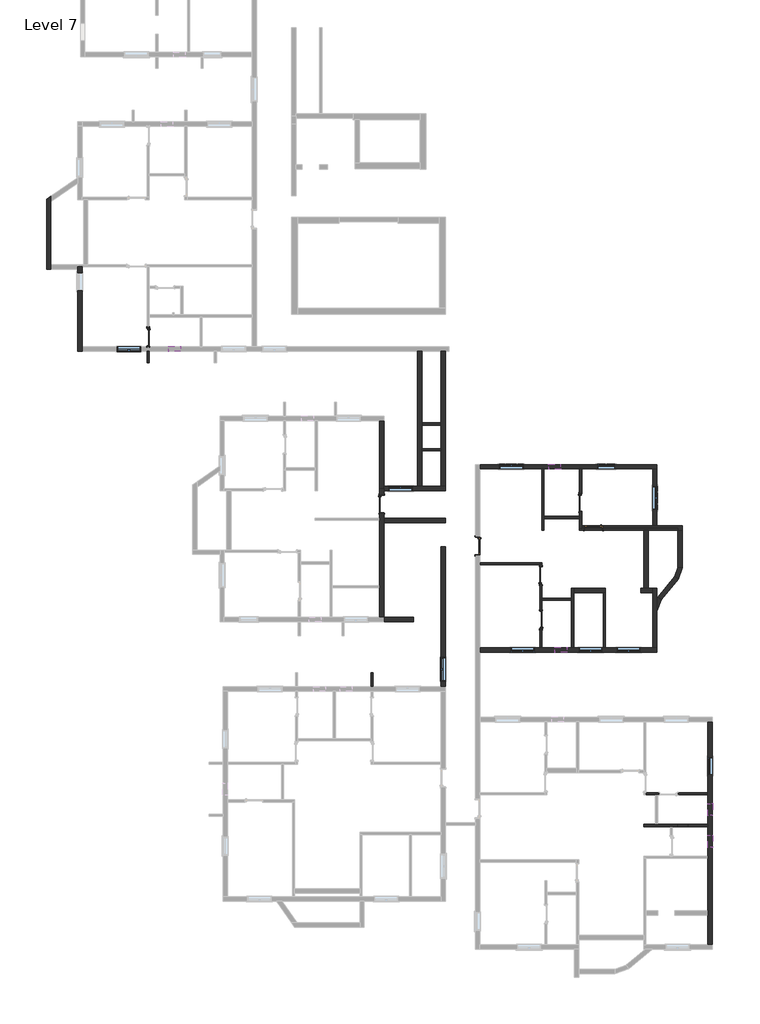
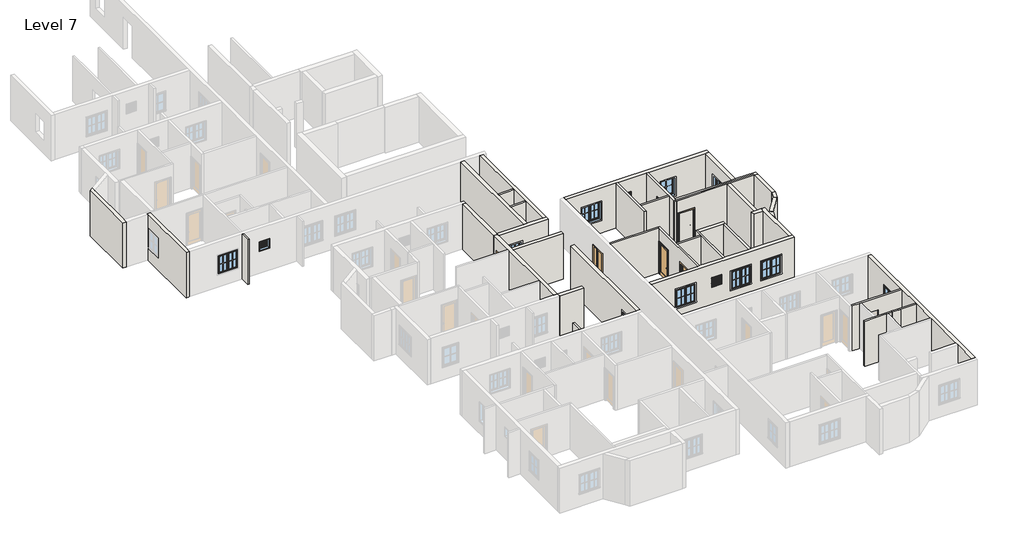
# One storey, part 3 of 7: 39 walls, 15 windows, 7 doors.
# Revit data of these elements (continued)
# Element 52 (IfcWindow, "Window-Casement-Double : 4' x 4'") (continued)
#   Interior Wall Closure = 0' - 2 1/4"
#   Frame Extension = 0' - 0 1/4"
#   Exterior Wall Closure = 0' - 1 1/4"
#   Interior Trim Visibility = yes
#   Exterior Trim Visibility = yes
#   Phase Created = New Construction
#   Materials on its faces: "Wood - Stained", "Glass", "Clad - White"
# Element 53 (IfcWindow, "Window-Casement-Double : 4' x 4'")
#   Mark = "176"
#   Window Inset = 0' - 0"
#   Interior Wall Closure = 0' - 2 1/4"
#   Frame Extension = 0' - 0 1/4"
#   Exterior Wall Closure = 0' - 1 1/4"
#   Interior Trim Visibility = yes
#   Exterior Trim Visibility = yes
#   Phase Created = New Construction
#   Materials on its faces: "Wood - Stained", "Glass", "Clad - White"
# Element 54 (IfcWindow, "Window-Casement-Double : 4' x 4'")
#   Mark = "187"
#   Window Inset = 0' - 0"
#   Interior Wall Closure = 0' - 2 1/4"
#   Frame Extension = 0' - 0 1/4"
#   Exterior Wall Closure = 0' - 1 1/4"
#   Interior Trim Visibility = yes
#   Exterior Trim Visibility = yes
#   Phase Created = New Construction
#   Materials on its faces: "Wood - Stained", "Glass", "Clad - White"
# Element 55 (IfcWindow, "Window-Casement-Double : 4' x 4'")
#   Mark = "190"
#   Window Inset = 0' - 0"
#   Interior Wall Closure = 0' - 2 1/4"
#   Frame Extension = 0' - 0 1/4"
#   Exterior Wall Closure = 0' - 1 1/4"
#   Interior Trim Visibility = yes
#   Exterior Trim Visibility = yes
#   Phase Created = New Construction
#   Materials on its faces: "Wood - Stained", "Glass", "Clad - White"
# Element 56 (IfcWindow, "Window-Casement-Double : 4' x 4'")
#   Mark = "195"
#   Window Inset = 0' - 0"
#   Interior Wall Closure = 0' - 2 1/4"
#   Frame Extension = 0' - 0 1/4"
#   Exterior Wall Closure = 0' - 1 1/4"
#   Interior Trim Visibility = yes
#   Exterior Trim Visibility = yes
#   Phase Created = New Construction
#   Materials on its faces: "Wood - Stained", "Glass", "Clad - White"
# Element 57 (IfcWindow, "Window-Louvers : 24\" x 24\"")
#   Mark = "138"
#   Blade Width = 1' - 10 1/2"
#   Phase Created = New Construction
#   Materials on its faces: "Birch"
# Element 58 (IfcWindow, "Window-Louvers : 24\" x 24\"")
#   Mark = "141"
#   Blade Width = 1' - 10 1/2"
#   Phase Created = New Construction
#   Materials on its faces: "Birch"
# Element 59 (IfcWindow, "Window-Louvers : 24\" x 24\"")
#   Mark = "142"
#   Blade Width = 1' - 10 1/2"
#   Phase Created = New Construction
#   Materials on its faces: "Birch"
# Element 60 (IfcWindow, "Window-Louvers : 24\" x 24\"")
#   Mark = "147"
#   Blade Width = 1' - 10 1/2"
#   Phase Created = New Construction
#   Materials on its faces: "Birch"
# Element 61 (IfcWindow, "Window-Louvers : 24\" x 24\"")
#   Mark = "148"
#   Blade Width = 1' - 10 1/2"
#   Phase Created = New Construction
#   Materials on its faces: "Birch"
# Materials
#   "Cherry": class "Wood", colour RGB 226 177 128, transparency 0, Description = "Prunus Serotina", Cost = 0
#   "Aluminum": class "Metal", colour RGB 247 247 247, transparency 0, Description = "Aluminum 6061", Cost = 0
#   "Wood - Stained": class "Wood", colour RGB 224 178 126, transparency 0, Cost = 0
#   "Glass": class "Glass", colour RGB 0 128 192, transparency 0.75, Description = "Soda Lime Glass", Cost = 0
#   "Clad - White": class "Wood", colour RGB 242 242 238, transparency 0, Cost = 0
#   "Birch": class "Wood", colour RGB 224 178 126, transparency 0, Description = "Betula Alleghaniensis", Cost = 0
#   "Default Wall": colour RGB 128 128 128, transparency 0, Cost = 0
